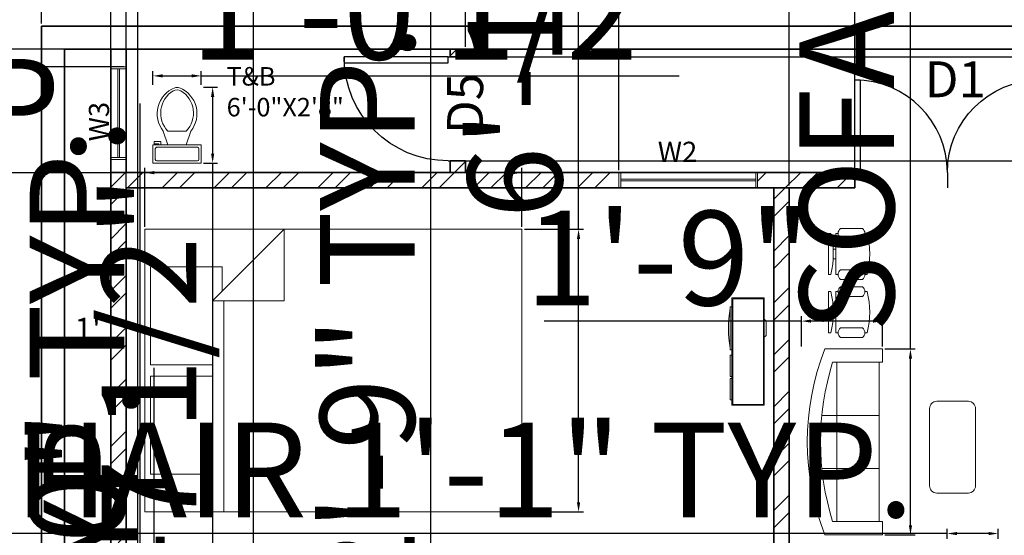
# Model space of a CAD drawing. Units: inches. Extents: x 1542 to 2523, y 1699 to 2449.
# Tile 4 of 7: x 1875 to 2130, y 2158 to 2292. Entities that reach past the tile are written whole.
import ezdxf

# ---------------------------------------------------------------- set-up
doc = ezdxf.new("R2010")
doc.units = ezdxf.units.IN
for name, color, linetype, lineweight in [('A-ANNO-DIMS', 7, 'Continuous', 18), ('A-ANNO-TEXT', 1, 'Continuous', 18), ('A-AREA-IDEN', 1, 'Continuous', 25), ('A-FLOR-FIXT', 9, 'Continuous', 18), ('A-WALL-PATT', 9, 'Continuous', 13), ('doors', 5, 'Continuous', 25), ('furniture', 9, 'Continuous', 18), ('walls', 7, 'Continuous', 35), ('windows', 93, 'Continuous', 18)]:
    doc.layers.add(name, color=color, linetype=linetype, lineweight=lineweight)
doc.styles.get("Standard").update_dxf_attribs({"font": 'arial.ttf'})
doc.dimstyles.new('ISO-25', dxfattribs={"dimtxt": 24.5625, "dimasz": 2.5, "dimexe": 1.25, "dimexo": 0.625, "dimtad": 1, "dimlunit": 4, "dimtxsty": 'Standard', "dimcen": 2.5, "dimadec": 0, "dimazin": 0, "dimtfac": 10, "dimtmove": 0, "dimatfit": 3, "dimfxl": 1, "dimarcsym": 0})

# ---------------------------------------------------------------- blocks, each defined once
blk = doc.blocks.new('*U2')
for p, q in [((0, 0), (0, -5)), ((30, 0), (30, -5))]:
    blk.add_line(p, q)
blk.add_lwpolyline([(0, 0), (0, 30), (1.75, 30), (1.75, 0)], close=True)
blk.add_arc((0, 0), 30, 0, 90)
blk = doc.blocks.new('Sofa - Roundback 7 ft.')
for p, q in [((-12.00002, -32.4421), (-12.00003, -6.5971)), ((11.99997, -32.4421), (11.99998, -6.5971)), ((-36.000027, -34), (-36.000027, -11.4696)), ((35.99998, -34), (35.99998, -11.4696)), ((-35.999844, -13.3819), (35.9998, -13.3819)), ((-36.000027, -32.4421), (35.99998, -32.4421))]:
    blk.add_line(p, q)
for points in [[(-36.000027, -34), (-42.000027, -34), (-42.000027, -8)], [(41.99998, -8), (41.99998, -34), (35.99998, -34)]]:
    blk.add_lwpolyline(points)
for centre, radius, start, end in [((0, -114.25), 114.25, 68.43141, 111.5686), ((-0.00001, -127.1968), 121.1968, 72.72033, 107.2797)]:
    blk.add_arc(centre, radius, start, end)
blk = doc.blocks.new('Bed - Queen')
for p, q in [((0, -80.00003), (0, 0)), ((0, 0), (59.99999, 0)), ((59.99999, 0), (59.99999, -80.00003)), ((7.99999, -1.2), (28.79998, -1.2)), ((7.99999, -14.4), (7.99999, -1.2)), ((28.79998, -1.2), (28.79998, -14.4)), ((31.19999, -1.2), (51.99999, -1.2)), ((31.19999, -14.4), (31.19999, -1.2)), ((51.99999, -1.2), (51.99999, -16.4)), ((0, -14.4), (44.8, -14.4)), ((59.99999, -29.6), (44.8, -14.4)), ((44.8, -14.4), (44.8, -29.6)), ((51.99999, -16.4), (46.79936, -16.4)), ((44.8, -16.8), (0, -16.8)), ((44.8, -29.6), (59.99999, -29.6)), ((59.99999, -80.00003), (0, -80.00003))]:
    blk.add_line(p, q)
blk = doc.blocks.new('Chair - Desk')
for p, q in [((-8.5, 0), (-8.5, -1)), ((-8.5, 0), (8.5, 0)), ((8.5, 0), (8.5, -1)), ((-8.5, -3), (-8.5, -4)), ((-8.5, -3), (8.5, -3)), ((-2, -3), (-2, -1.9355)), ((2, -1.9576), (2, -3)), ((8.5, -3), (8.5, -4)), ((-10.5, -5), (-10.5, -14)), ((-6.5, -14), (-6.5, -5)), ((6.5, -5), (6.5, -14)), ((10.5, -14), (10.5, -5)), ((-8.5, -15), (-8.5, -16)), ((8.5, -15), (8.5, -16))]:
    blk.add_line(p, q)
for centre, radius, start, end in [((-8.5, -6.5), 2.5, 36.8699, 143.1301), ((0, 34.625), 36.625, 256.5803, 283.4197), ((8.5, -6.5), 2.5, 36.8699, 143.1301), ((-8.5, -12.5), 2.5, 216.8699, 323.1301), ((0, 19.625), 36.625, 256.5803, 283.4197), ((8.5, -12.5), 2.5, 216.8699, 323.1301)]:
    blk.add_arc(centre, radius, start, end)
blk = doc.blocks.new('Entertainment Center')
for p, q in [((-4, 0), (-5, -1)), ((4, 0), (-4, 0)), ((5, -1), (4, 0)), ((-17, -19), (-17, -1)), ((-17, -1), (43, -1)), ((-16.5, -18.5), (-16.5, -1.5)), ((-16.5, -1.5), (42.5, -1.5)), ((42.5, -1.5), (42.5, -18.5)), ((43, -1), (43, -19)), ((43, -19), (-17, -19)), ((42.5, -18.5), (-16.5, -18.5)), ((-12, -20), (-12, -19)), ((12, -20), (-12, -20)), ((12, -19), (12, -20)), ((15, -20), (15, -19)), ((27, -20), (15, -20)), ((27, -19), (27, -20)), ((28, -20), (28, -19)), ((40, -20), (28, -20)), ((40, -19), (40, -20))]:
    blk.add_line(p, q)
blk.add_arc((0, 40), 61, 259.6111, 280.3889)
blk = doc.blocks.new('Toilet - top')
for p, q in [((9.5, -6), (9.5, -2)), ((-10, -8.5), (-8, -8.5)), ((-10, -9.5), (-10, -8.5)), ((-8, -8.5), (-8, -8)), ((-7, -8), (-7, -9.5)), ((-4, -8), (-6, -14)), ((4, -8), (6, -14)), ((-7, -9.5), (-10, -9.5)), ((4, -14), (-4, -14))]:
    blk.add_line(p, q)
blk.add_lwpolyline([(10.5, -8), (10.5, 0), (-10.5, 0), (-10.5, -8)], close=True)
for points in [[(-9.5, -2), (-9.5, -6)], [(8.5, -1), (-8.5, -1)], [(-8.5, -7), (8.5, -7)]]:
    blk.add_lwpolyline(points)
for centre, radius, start, end in [((-8.62, -1.88), 0.884, 81.8699, 188.1301), ((8.62, -1.88), 0.884, 351.8699, 98.1301), ((-8.62, -6.12), 0.884, 171.8699, 278.1301), ((8.62, -6.12), 0.884, 261.8699, 8.1301), ((3.52, -21.58), 12.17, 141.4691, 247.9714), ((4.2, -21.82), 11.33, 136.3677, 238.9468), ((-3.52, -21.58), 12.17, 292.0284, 38.5307), ((-4.2, -21.82), 11.33, 301.053, 43.6321), ((0, -27.88), 4, 245.7318, 294.2682), ((0, -29), 4, 254.8605, 285.1395)]:
    blk.add_arc(centre, radius, start, end)
blk = doc.blocks.new('*D9')
at = {"layer": 'A-ANNO-DIMS', "color": 0, "lineweight": -2, "transparency": 16777216}
for p, q in [((1880.38, 2291.06), (1880.38, 2302.87)), ((1882.88, 2301.62), (2237.88, 2301.62)), ((2240.38, 2291.06), (2240.38, 2302.87))]:
    blk.add_line(p, q, dxfattribs=at)
at = {"layer": 'A-ANNO-DIMS', "color": 0, "transparency": 16777216}
for points in [[(1882.88, 2302.04), (1882.88, 2301.2), (1880.38, 2301.62)], [(2237.88, 2302.04), (2237.88, 2301.2), (2240.38, 2301.62)]]:
    blk.add_solid(points, dxfattribs=at)
at = {"layer": 'Defpoints', "color": 0, "transparency": 16777216}
for p in [(2240.38, 2301.62), (1880.38, 2290.44), (2240.38, 2290.44)]:
    blk.add_point(p, dxfattribs=at)
at = {"layer": 'A-ANNO-DIMS', "color": 0, "transparency": 16777216, "insert": (2060.38, 2308.37), "char_height": 12, "attachment_point": 5}
blk.add_mtext("30'", dxfattribs=at)
blk = doc.blocks.new('*D17')
at = {"layer": 'A-ANNO-DIMS', "color": 0, "lineweight": -2, "transparency": 16777216}
for p, q in [((1886.38, 2206.47), (1886.38, 2208.52)), ((1895.88, 2207.27), (1888.88, 2207.27)), ((1898.38, 2206.47), (1898.38, 2208.52))]:
    blk.add_line(p, q, dxfattribs=at)
at = {"layer": 'A-ANNO-DIMS', "color": 0, "transparency": 16777216}
for points in [[(1888.88, 2207.69), (1888.88, 2206.86), (1886.38, 2207.27)], [(1895.88, 2207.69), (1895.88, 2206.86), (1898.38, 2207.27)]]:
    blk.add_solid(points, dxfattribs=at)
at = {"layer": 'Defpoints', "color": 0, "transparency": 16777216}
for p in [(1886.38, 2207.27), (1886.38, 2205.84), (1898.38, 2205.84)]:
    blk.add_point(p, dxfattribs=at)
at = {"layer": 'A-ANNO-DIMS', "color": 0, "transparency": 16777216, "insert": (1892.38, 2210.91), "char_height": 6, "attachment_point": 5}
blk.add_mtext("1'", dxfattribs=at)
blk = doc.blocks.new('WIN-W3-24IN')
for p, q in [((0, 0), (0, 24.03)), ((0, 24.03), (3.94, 24.03)), ((0, 23.53), (3.94, 23.53)), ((1.77, 0.5), (1.77, 23.53)), ((2.17, 0.5), (2.17, 23.53)), ((3.94, 24.03), (3.94, 0)), ((3.94, 0.5), (0, 0.5)), ((3.94, 0), (0, 0))]:
    blk.add_line(p, q)
blk = doc.blocks.new('WIN-W2-36IN')
for p, q in [((0, 3.94), (36.03, 3.94)), ((0, 0), (0, 3.94)), ((0.5, 0), (0.5, 3.94)), ((35.53, 3.94), (35.53, 0)), ((36.03, 3.94), (36.03, 0)), ((36.03, 0), (0, 0)), ((0.5, 2.17), (35.53, 2.17)), ((0.5, 1.77), (35.53, 1.77))]:
    blk.add_line(p, q)
blk = doc.blocks.new('*D26')
at = {"layer": 'A-ANNO-DIMS', "color": 0, "lineweight": -2, "transparency": 16777216}
for p, q in [((2115.34, 2158.69), (1845.86, 2158.69)), ((2115.34, 2157.33), (2115.34, 2159.94)), ((2126.05, 2158.69), (2117.84, 2158.69)), ((2128.55, 2157.33), (2128.55, 2159.94))]:
    blk.add_line(p, q, dxfattribs=at)
at = {"layer": 'A-ANNO-DIMS', "color": 0, "transparency": 16777216}
for points in [[(2117.84, 2159.1), (2117.84, 2158.27), (2115.34, 2158.69)], [(2126.05, 2159.1), (2126.05, 2158.27), (2128.55, 2158.69)]]:
    blk.add_solid(points, dxfattribs=at)
at = {"layer": 'Defpoints', "color": 0, "transparency": 16777216}
for p in [(2115.34, 2158.69), (2115.34, 2156.7), (2128.55, 2156.7)]:
    blk.add_point(p, dxfattribs=at)
at = {"layer": 'A-ANNO-DIMS', "color": 0, "transparency": 16777216, "insert": (1979.35, 2172.01), "char_height": 24.5625, "attachment_point": 5}
blk.add_mtext('CHAIR 1\'-1" TYP.', dxfattribs=at)
blk = doc.blocks.new('*D28')
at = {"layer": 'A-ANNO-DIMS', "color": 0, "lineweight": -2, "transparency": 16777216}
for p, q in [((1905.99, 2054.87), (1905.99, 2270.35)), ((1903.01, 2054.87), (1907.24, 2054.87)), ((1905.99, 2033.33), (1905.99, 2052.37)), ((1903.01, 2030.83), (1907.24, 2030.83))]:
    blk.add_line(p, q, dxfattribs=at)
at = {"layer": 'A-ANNO-DIMS', "color": 0, "transparency": 16777216}
for points in [[(1905.57, 2052.37), (1906.4, 2052.37), (1905.99, 2054.87)], [(1905.57, 2033.33), (1906.4, 2033.33), (1905.99, 2030.83)]]:
    blk.add_solid(points, dxfattribs=at)
at = {"layer": 'Defpoints', "color": 0, "transparency": 16777216}
for p in [(1902.38, 2054.87), (1905.99, 2054.87), (1902.38, 2030.83)]:
    blk.add_point(p, dxfattribs=at)
at = {"layer": 'A-ANNO-DIMS', "color": 0, "transparency": 16777216, "insert": (1892.81, 2163.86), "char_height": 24.5625, "attachment_point": 5, "rotation": 90}
blk.add_mtext('W3 2\'-0" TYP.', dxfattribs=at)
blk = doc.blocks.new('*D30')
at = {"layer": 'A-ANNO-DIMS', "color": 0, "lineweight": -2, "transparency": 16777216}
for p, q in [((2181.19, 2203.89), (2176.38, 2203.89)), ((2177.63, 2201.39), (2177.63, 2178.49)), ((2181.19, 2175.99), (2176.38, 2175.99)), ((2177.63, 2175.99), (2177.63, 1878.93))]:
    blk.add_line(p, q, dxfattribs=at)
at = {"layer": 'A-ANNO-DIMS', "color": 0, "transparency": 16777216}
for points in [[(2177.21, 2201.39), (2178.05, 2201.39), (2177.63, 2203.89)], [(2177.21, 2178.49), (2178.05, 2178.49), (2177.63, 2175.99)]]:
    blk.add_solid(points, dxfattribs=at)
at = {"layer": 'Defpoints', "color": 0, "transparency": 16777216}
for p in [(2181.81, 2203.89), (2177.63, 2175.99), (2181.81, 2175.99)]:
    blk.add_point(p, dxfattribs=at)
at = {"layer": 'A-ANNO-DIMS', "color": 0, "transparency": 16777216, "insert": (2164.46, 2026.21), "char_height": 24.5625, "attachment_point": 5, "rotation": 90}
blk.add_mtext('TV UNIT 2\'-4" TYP.', dxfattribs=at)
blk = doc.blocks.new('*D32')
at = {"layer": 'A-ANNO-DIMS', "color": 0, "lineweight": -2, "transparency": 16777216}
for p, q in [((1922.46, 2274.54), (1926.04, 2274.54)), ((1924.79, 2272.04), (1924.79, 2257.33)), ((1922.46, 2254.83), (1926.04, 2254.83)), ((1924.79, 2254.83), (1924.79, 2060.84))]:
    blk.add_line(p, q, dxfattribs=at)
at = {"layer": 'A-ANNO-DIMS', "color": 0, "transparency": 16777216}
for points in [[(1924.37, 2272.04), (1925.21, 2272.04), (1924.79, 2274.54)], [(1924.37, 2257.33), (1925.21, 2257.33), (1924.79, 2254.83)]]:
    blk.add_solid(points, dxfattribs=at)
at = {"layer": 'Defpoints', "color": 0, "transparency": 16777216}
for p in [(1921.83, 2274.54), (1921.83, 2254.83), (1924.79, 2254.83)]:
    blk.add_point(p, dxfattribs=at)
at = {"layer": 'A-ANNO-DIMS', "color": 0, "transparency": 16777216, "insert": (1911.46, 2156.58), "char_height": 24.5625, "attachment_point": 5, "rotation": 90}
blk.add_mtext('WC 1\'-7 1/2"', dxfattribs=at)
blk = doc.blocks.new('*D33')
at = {"layer": 'A-ANNO-DIMS', "color": 0, "lineweight": -2, "transparency": 16777216}
for p, q in [((1909.3, 2275.17), (1909.3, 2278.75)), ((1921.83, 2275.17), (1921.83, 2278.75)), ((1911.8, 2277.5), (1919.33, 2277.5)), ((1921.83, 2277.5), (2045.8, 2277.5))]:
    blk.add_line(p, q, dxfattribs=at)
at = {"layer": 'A-ANNO-DIMS', "color": 0, "transparency": 16777216}
for points in [[(1911.8, 2277.92), (1911.8, 2277.09), (1909.3, 2277.5)], [(1919.33, 2277.92), (1919.33, 2277.09), (1921.83, 2277.5)]]:
    blk.add_solid(points, dxfattribs=at)
at = {"layer": 'Defpoints', "color": 0, "transparency": 16777216}
for p in [(1921.83, 2277.5), (1909.3, 2274.54), (1921.83, 2274.54)]:
    blk.add_point(p, dxfattribs=at)
at = {"layer": 'A-ANNO-DIMS', "color": 0, "transparency": 16777216, "insert": (1985.06, 2290.83), "char_height": 24.562, "attachment_point": 5}
blk.add_mtext('1\'-0 1/2"', dxfattribs=at)
blk = doc.blocks.new('*D34')
at = {"layer": 'A-ANNO-DIMS', "color": 0, "lineweight": -2, "transparency": 16777216}
for p, q in [((1981.43, 2074.83), (1981.43, 2296.01)), ((1977.09, 2074.83), (1982.68, 2074.83)), ((1981.43, 2044.29), (1981.43, 2072.33)), ((1977.09, 2041.79), (1982.68, 2041.79))]:
    blk.add_line(p, q, dxfattribs=at)
at = {"layer": 'A-ANNO-DIMS', "color": 0, "transparency": 16777216}
for points in [[(1981.01, 2072.33), (1981.84, 2072.33), (1981.43, 2074.83)], [(1981.01, 2044.29), (1981.84, 2044.29), (1981.43, 2041.79)]]:
    blk.add_solid(points, dxfattribs=at)
at = {"layer": 'Defpoints', "color": 0, "transparency": 16777216}
for p in [(1976.47, 2074.83), (1981.43, 2074.83), (1976.47, 2041.79)]:
    blk.add_point(p, dxfattribs=at)
at = {"layer": 'A-ANNO-DIMS', "color": 0, "transparency": 16777216, "insert": (1968.1, 2186.67), "char_height": 24.5625, "attachment_point": 5, "rotation": 90}
blk.add_mtext('WC 2\'-9" TYP.', dxfattribs=at)
blk = doc.blocks.new('*D38')
at = {"layer": 'A-ANNO-DIMS', "color": 0, "lineweight": -2, "transparency": 16777216}
for p, q in [((1907.17, 2238.32), (1907.17, 2253.62)), ((2005.03, 2238.32), (2005.03, 2253.62)), ((1907.17, 2252.37), (1542.11, 2252.37)), ((2002.53, 2252.37), (1909.67, 2252.37))]:
    blk.add_line(p, q, dxfattribs=at)
at = {"layer": 'A-ANNO-DIMS', "color": 0, "transparency": 16777216}
for points in [[(1909.67, 2252.79), (1909.67, 2251.95), (1907.17, 2252.37)], [(2002.53, 2252.79), (2002.53, 2251.95), (2005.03, 2252.37)]]:
    blk.add_solid(points, dxfattribs=at)
at = {"layer": 'Defpoints', "color": 0, "transparency": 16777216}
for p in [(1907.17, 2252.37), (1907.17, 2237.69), (2005.03, 2237.69)]:
    blk.add_point(p, dxfattribs=at)
at = {"layer": 'A-ANNO-DIMS', "color": 0, "transparency": 16777216, "insert": (1723.39, 2266.45), "char_height": 24.5625, "attachment_point": 5}
blk.add_mtext('QUEEN BED 8\'-2" TYP.', dxfattribs=at)
blk = doc.blocks.new('*D39')
at = {"layer": 'A-ANNO-DIMS', "color": 0, "lineweight": -2, "transparency": 16777216}
for p, q in [((2019.71, 2237.69), (2019.71, 2448.53)), ((2005.65, 2237.69), (2020.96, 2237.69)), ((2019.71, 2166.8), (2019.71, 2235.19)), ((2005.65, 2164.3), (2020.96, 2164.3))]:
    blk.add_line(p, q, dxfattribs=at)
at = {"layer": 'A-ANNO-DIMS', "color": 0, "transparency": 16777216}
for points in [[(2019.29, 2235.19), (2020.12, 2235.19), (2019.71, 2237.69)], [(2019.29, 2166.8), (2020.12, 2166.8), (2019.71, 2164.3)]]:
    blk.add_solid(points, dxfattribs=at)
at = {"layer": 'Defpoints', "color": 0, "transparency": 16777216}
for p in [(2005.03, 2237.69), (2019.71, 2237.69), (2005.03, 2164.3)]:
    blk.add_point(p, dxfattribs=at)
at = {"layer": 'A-ANNO-DIMS', "color": 0, "transparency": 16777216, "insert": (2006.38, 2344.36), "char_height": 24.5625, "attachment_point": 5, "rotation": 90}
blk.add_mtext('6\'-1 1/2" TYP.', dxfattribs=at)
blk = doc.blocks.new('*D40')
at = {"layer": 'A-ANNO-DIMS', "color": 0, "lineweight": -2, "transparency": 16777216}
for p, q in [((1909.59, 1986.22), (1909.59, 2201.7)), ((1903.01, 1986.22), (1910.84, 1986.22)), ((1909.59, 1940.69), (1909.59, 1983.72)), ((1903.01, 1938.19), (1910.84, 1938.19))]:
    blk.add_line(p, q, dxfattribs=at)
at = {"layer": 'A-ANNO-DIMS', "color": 0, "transparency": 16777216}
for points in [[(1909.17, 1983.72), (1910, 1983.72), (1909.59, 1986.22)], [(1909.17, 1940.69), (1910, 1940.69), (1909.59, 1938.19)]]:
    blk.add_solid(points, dxfattribs=at)
at = {"layer": 'Defpoints', "color": 0, "transparency": 16777216}
for p in [(1902.38, 1986.22), (1909.59, 1986.22), (1902.38, 1938.19)]:
    blk.add_point(p, dxfattribs=at)
at = {"layer": 'A-ANNO-DIMS', "color": 0, "transparency": 16777216, "insert": (1896.42, 2095.21), "char_height": 24.5625, "attachment_point": 5, "rotation": 90}
blk.add_mtext('W1 4\'-0" TYP.', dxfattribs=at)
blk = doc.blocks.new('*D44')
at = {"layer": 'A-ANNO-DIMS', "color": 0, "lineweight": -2, "transparency": 16777216}
for p, q in [((2105.8, 2206.61), (2105.8, 2435.72)), ((2099.19, 2206.61), (2107.05, 2206.61)), ((2105.8, 2160.85), (2105.8, 2204.11)), ((2099.19, 2158.35), (2107.05, 2158.35))]:
    blk.add_line(p, q, dxfattribs=at)
at = {"layer": 'A-ANNO-DIMS', "color": 0, "transparency": 16777216}
for points in [[(2105.39, 2204.11), (2106.22, 2204.11), (2105.8, 2206.61)], [(2105.39, 2160.85), (2106.22, 2160.85), (2105.8, 2158.35)]]:
    blk.add_solid(points, dxfattribs=at)
at = {"layer": 'Defpoints', "color": 0, "transparency": 16777216}
for p in [(2098.56, 2206.61), (2105.8, 2206.61), (2098.56, 2158.35)]:
    blk.add_point(p, dxfattribs=at)
at = {"layer": 'A-ANNO-DIMS', "color": 0, "transparency": 16777216, "insert": (2092.47, 2322.42), "char_height": 24.5625, "attachment_point": 5, "rotation": 90}
blk.add_mtext('SOFA 4\'-0 1/2"', dxfattribs=at)
blk = doc.blocks.new('*D45')
at = {"layer": 'A-ANNO-DIMS', "color": 0, "lineweight": -2, "transparency": 16777216}
for p, q in [((2077.5, 2207.23), (2077.5, 2215.09)), ((2098.56, 2207.23), (2098.56, 2215.09)), ((2077.5, 2213.84), (2010.77, 2213.84)), ((2096.06, 2213.84), (2080, 2213.84))]:
    blk.add_line(p, q, dxfattribs=at)
at = {"layer": 'A-ANNO-DIMS', "color": 0, "transparency": 16777216}
for points in [[(2080, 2214.26), (2080, 2213.43), (2077.5, 2213.84)], [(2096.06, 2214.26), (2096.06, 2213.43), (2098.56, 2213.84)]]:
    blk.add_solid(points, dxfattribs=at)
at = {"layer": 'Defpoints', "color": 0, "transparency": 16777216}
for p in [(2077.5, 2213.84), (2077.5, 2206.61), (2098.56, 2206.61)]:
    blk.add_point(p, dxfattribs=at)
at = {"layer": 'A-ANNO-DIMS', "color": 0, "transparency": 16777216, "insert": (2042.89, 2227.01), "char_height": 24.562, "attachment_point": 5}
blk.add_mtext('1\'-9"', dxfattribs=at)
blk = doc.blocks.new('*D48')
at = {"layer": 'A-ANNO-DIMS', "color": 0, "lineweight": -2, "transparency": 16777216}
for p, q in [((1905.38, 2077.06), (1905.38, 2320.14)), ((1935.38, 2077.06), (1935.38, 2320.14)), ((1907.88, 2318.89), (1932.88, 2318.89)), ((1935.38, 2318.89), (2004.84, 2318.89))]:
    blk.add_line(p, q, dxfattribs=at)
at = {"layer": 'A-ANNO-DIMS', "color": 0, "transparency": 16777216}
for points in [[(1907.88, 2319.31), (1907.88, 2318.47), (1905.38, 2318.89)], [(1932.88, 2319.31), (1932.88, 2318.47), (1935.38, 2318.89)]]:
    blk.add_solid(points, dxfattribs=at)
at = {"layer": 'Defpoints', "color": 0, "transparency": 16777216}
for p in [(1935.38, 2318.89), (1905.38, 2076.44), (1935.38, 2076.44)]:
    blk.add_point(p, dxfattribs=at)
at = {"layer": 'A-ANNO-DIMS', "color": 0, "transparency": 16777216, "insert": (1971.36, 2332.05), "char_height": 24.562, "attachment_point": 5}
blk.add_mtext('2\'-6"', dxfattribs=at)
blk = doc.blocks.new('*D50')
at = {"layer": 'A-ANNO-DIMS', "color": 0, "lineweight": -2, "transparency": 16777216}
for p, q in [((2268.83, 2282.44), (2268.83, 2351.9)), ((1987.01, 2282.44), (2270.08, 2282.44)), ((2268.83, 2257.94), (2268.83, 2279.94)), ((1987.01, 2255.44), (2270.08, 2255.44))]:
    blk.add_line(p, q, dxfattribs=at)
at = {"layer": 'A-ANNO-DIMS', "color": 0, "transparency": 16777216}
for points in [[(2268.42, 2279.94), (2269.25, 2279.94), (2268.83, 2282.44)], [(2268.42, 2257.94), (2269.25, 2257.94), (2268.83, 2255.44)]]:
    blk.add_solid(points, dxfattribs=at)
at = {"layer": 'Defpoints', "color": 0, "transparency": 16777216}
for p in [(1986.38, 2282.44), (2268.83, 2282.44), (1986.38, 2255.44)]:
    blk.add_point(p, dxfattribs=at)
at = {"layer": 'A-ANNO-DIMS', "color": 0, "transparency": 16777216, "insert": (2255.66, 2318.42), "char_height": 24.562, "attachment_point": 5, "rotation": 90}
blk.add_mtext('2\'-3"', dxfattribs=at)
blk = doc.blocks.new('*D57')
at = {"layer": 'A-ANNO-DIMS', "color": 0, "lineweight": -2, "transparency": 16777216}
for p, q in [((1851.93, 2089.65), (1851.93, 2178.19)), ((1897.82, 2089.65), (1850.68, 2089.65)), ((1851.93, 2057.37), (1851.93, 2087.15)), ((1897.82, 2054.87), (1850.68, 2054.87))]:
    blk.add_line(p, q, dxfattribs=at)
at = {"layer": 'A-ANNO-DIMS', "color": 0, "transparency": 16777216}
for points in [[(1851.52, 2087.15), (1852.35, 2087.15), (1851.93, 2089.65)], [(1851.52, 2057.37), (1852.35, 2057.37), (1851.93, 2054.87)]]:
    blk.add_solid(points, dxfattribs=at)
at = {"layer": 'Defpoints', "color": 0, "transparency": 16777216}
for p in [(1851.93, 2089.65), (1898.45, 2089.65), (1898.45, 2054.87)]:
    blk.add_point(p, dxfattribs=at)
at = {"layer": 'A-ANNO-DIMS', "color": 0, "transparency": 16777216, "insert": (1838.98, 2135.17), "char_height": 24.562, "attachment_point": 5, "rotation": 90}
blk.add_mtext('2\'-11"', dxfattribs=at)
blk = doc.blocks.new('*D61')
at = {"layer": 'A-ANNO-DIMS', "color": 0, "lineweight": -2, "transparency": 16777216}
for p, q in [((1898.38, 2253.06), (1898.38, 2320.14)), ((2030.14, 2253.06), (2030.14, 2320.14)), ((1900.88, 2318.89), (2027.64, 2318.89))]:
    blk.add_line(p, q, dxfattribs=at)
at = {"layer": 'A-ANNO-DIMS', "color": 0, "transparency": 16777216}
for points in [[(1900.88, 2319.31), (1900.88, 2318.47), (1898.38, 2318.89)], [(2027.64, 2319.31), (2027.64, 2318.47), (2030.14, 2318.89)]]:
    blk.add_solid(points, dxfattribs=at)
at = {"layer": 'Defpoints', "color": 0, "transparency": 16777216}
for p in [(2030.14, 2318.89), (1898.38, 2252.44), (2030.14, 2252.44)]:
    blk.add_point(p, dxfattribs=at)
at = {"layer": 'A-ANNO-DIMS', "color": 0, "transparency": 16777216, "insert": (1964.26, 2332.05), "char_height": 24.562, "attachment_point": 5}
blk.add_mtext('11\'-0"', dxfattribs=at)
blk = doc.blocks.new('*D62')
at = {"layer": 'A-ANNO-DIMS', "color": 0, "lineweight": -2, "transparency": 16777216}
for p, q in [((2074.38, 2249.06), (2074.38, 2320.14)), ((2091.38, 2249.06), (2091.38, 2320.14)), ((2076.88, 2318.89), (2088.88, 2318.89)), ((2091.38, 2318.89), (2158.11, 2318.89))]:
    blk.add_line(p, q, dxfattribs=at)
at = {"layer": 'A-ANNO-DIMS', "color": 0, "transparency": 16777216}
for points in [[(2076.88, 2319.31), (2076.88, 2318.47), (2074.38, 2318.89)], [(2088.88, 2319.31), (2088.88, 2318.47), (2091.38, 2318.89)]]:
    blk.add_solid(points, dxfattribs=at)
at = {"layer": 'Defpoints', "color": 0, "transparency": 16777216}
for p in [(2091.38, 2318.89), (2074.38, 2248.44), (2091.38, 2248.44)]:
    blk.add_point(p, dxfattribs=at)
at = {"layer": 'A-ANNO-DIMS', "color": 0, "transparency": 16777216, "insert": (2126, 2332.05), "char_height": 24.562, "attachment_point": 5}
blk.add_mtext('1\'-5"', dxfattribs=at)
blk = doc.blocks.new('*D65')
at = {"layer": 'A-ANNO-DIMS', "color": 0, "lineweight": -2, "transparency": 16777216}
for p, q in [((1898.38, 2285.06), (1898.38, 2320.14)), ((1990.38, 2285.06), (1990.38, 2320.14)), ((1900.88, 2318.89), (1987.88, 2318.89))]:
    blk.add_line(p, q, dxfattribs=at)
at = {"layer": 'A-ANNO-DIMS', "color": 0, "transparency": 16777216}
for points in [[(1900.88, 2319.31), (1900.88, 2318.47), (1898.38, 2318.89)], [(1987.88, 2319.31), (1987.88, 2318.47), (1990.38, 2318.89)]]:
    blk.add_solid(points, dxfattribs=at)
at = {"layer": 'Defpoints', "color": 0, "transparency": 16777216}
for p in [(1990.38, 2318.89), (1898.38, 2284.44), (1990.38, 2284.44)]:
    blk.add_point(p, dxfattribs=at)
at = {"layer": 'A-ANNO-DIMS', "color": 0, "transparency": 16777216, "insert": (1944.38, 2332.05), "char_height": 24.562, "attachment_point": 5}
blk.add_mtext('7\'-8"', dxfattribs=at)
blk = doc.blocks.new('*D66')
at = {"layer": 'A-ANNO-DIMS', "color": 0, "lineweight": -2, "transparency": 16777216}
for p, q in [((1851.93, 2286.94), (1851.93, 2413.22)), ((1901.76, 2284.44), (1850.68, 2284.44)), ((1851.93, 2279.86), (1851.93, 2284.44)), ((1901.76, 2279.86), (1850.68, 2279.86)), ((1851.93, 2277.36), (1851.93, 2274.86))]:
    blk.add_line(p, q, dxfattribs=at)
at = {"layer": 'A-ANNO-DIMS', "color": 0, "transparency": 16777216}
for points in [[(1851.52, 2286.94), (1852.35, 2286.94), (1851.93, 2284.44)], [(1851.52, 2277.36), (1852.35, 2277.36), (1851.93, 2279.86)]]:
    blk.add_solid(points, dxfattribs=at)
at = {"layer": 'Defpoints', "color": 0, "transparency": 16777216}
for p in [(1851.93, 2284.44), (1902.38, 2284.44), (1902.38, 2279.86)]:
    blk.add_point(p, dxfattribs=at)
at = {"layer": 'A-ANNO-DIMS', "color": 0, "transparency": 16777216, "insert": (1838.61, 2351.33), "char_height": 24.562, "attachment_point": 5, "rotation": 90}
blk.add_mtext('0\'-4 1/2"', dxfattribs=at)
blk = doc.blocks.new('*D69')
at = {"layer": 'A-ANNO-DIMS', "color": 0, "lineweight": -2, "transparency": 16777216}
for p, q in [((1902.38, 2077.06), (1902.38, 2320.14)), ((1905.38, 2077.06), (1905.38, 2320.14)), ((1899.88, 2318.89), (1897.38, 2318.89)), ((1902.38, 2318.89), (1905.38, 2318.89)), ((1907.88, 2318.89), (1976.93, 2318.89))]:
    blk.add_line(p, q, dxfattribs=at)
at = {"layer": 'A-ANNO-DIMS', "color": 0, "transparency": 16777216}
for points in [[(1899.88, 2319.31), (1899.88, 2318.47), (1902.38, 2318.89)], [(1907.88, 2319.31), (1907.88, 2318.47), (1905.38, 2318.89)]]:
    blk.add_solid(points, dxfattribs=at)
at = {"layer": 'Defpoints', "color": 0, "transparency": 16777216}
for p in [(1905.38, 2318.89), (1902.38, 2076.44), (1905.38, 2076.44)]:
    blk.add_point(p, dxfattribs=at)
at = {"layer": 'A-ANNO-DIMS', "color": 0, "transparency": 16777216, "insert": (1943.65, 2332.06), "char_height": 24.562, "attachment_point": 5}
blk.add_mtext('0\'-3"', dxfattribs=at)

msp = doc.modelspace()

# ---------------------------------------------------------------- hatches: boundary and pattern name
at = {"layer": 'A-WALL-PATT'}
h = msp.add_hatch(dxfattribs=at)
h.set_pattern_fill('ANSI32', color=256)
h.paths.add_polyline_path([(1902.383, 2284.439), (1898.383, 2284.439), (1898.383, 2252.439), (1902.383, 2252.439), (1902.383, 2255.826), (1898.446, 2255.826), (1898.446, 2279.859), (1902.383, 2279.859)])
h = msp.add_hatch(dxfattribs=at)
h.set_pattern_fill('ANSI32', color=256)
h.paths.add_polyline_path([(1990.383, 2282.439), (1990.383, 2284.439), (1986.383, 2284.439), (1986.383, 2282.439)])
h = msp.add_hatch(dxfattribs=at)
h.set_pattern_fill('ANSI32', color=256)
h.paths.add_polyline_path([(1902.383, 2255.826), (1898.383, 2255.826), (1898.383, 2252.439), (1902.383, 2252.439)], flags=17)
h = msp.add_hatch(dxfattribs=at)
h.set_pattern_fill('ANSI32', color=256)
h.paths.add_polyline_path([(1990.383, 2255.439), (1986.383, 2255.439), (1986.383, 2252.439), (1990.383, 2252.439)])
h = msp.add_hatch(dxfattribs=at)
h.set_pattern_fill('ANSI32', color=256)
h.paths.add_polyline_path([(1902.383, 2125.681), (1898.383, 2125.681), (1898.383, 2252.439), (2030.138, 2252.439), (2030.138, 2248.439), (1902.383, 2248.439)])
h = msp.add_hatch(dxfattribs=at)
h.set_pattern_fill('ANSI32', color=256)
h.paths.add_polyline_path([(2091.383, 2252.439), (2066.17, 2252.439), (2066.17, 2248.439), (2091.383, 2248.439)])
h = msp.add_hatch(dxfattribs=at)
h.set_pattern_fill('ANSI32', color=256)
h.paths.add_polyline_path([(2074.383, 2248.439), (2070.383, 2248.439), (2070.383, 2119.439), (2074.383, 2119.439)])

# ---------------------------------------------------------------- linework, layer by layer
at = {"layer": 'furniture'}
msp.add_lwpolyline([(2110.762, 2191.173, -0.4142136), (2112.613, 2193.025), (2120.82, 2193.025, -0.4142136), (2122.671, 2191.173), (2122.671, 2171.058, -0.4142136), (2120.82, 2169.206), (2112.613, 2169.206, -0.4142136), (2110.762, 2171.058)], format="xyb", close=True, dxfattribs=at)
at = {"layer": 'walls'}
for p, q in [((1880.383, 2290.439), (2240.383, 2290.439)), ((1880.383, 1750.439), (1880.383, 2290.439)), ((1886.383, 2284.439), (2234.383, 2284.439)), ((1886.383, 1756.439), (1886.383, 2284.439)), ((1898.383, 2252.439), (1898.383, 2284.439)), ((1902.383, 2252.439), (1902.383, 2284.439)), ((1986.383, 2282.439), (1986.383, 2284.439)), ((1990.383, 2284.439), (1990.383, 2282.439)), ((1990.383, 2282.439), (1990.383, 2284.439)), ((1990.383, 2282.439), (1986.383, 2282.439)), ((1986.383, 2252.439), (1986.383, 2255.439)), ((1986.383, 2255.439), (1990.383, 2255.439)), ((1990.383, 2252.439), (1990.383, 2255.439)), ((1898.383, 1840.439), (1898.383, 2252.439)), ((2091.383, 2252.439), (1898.383, 2252.439)), ((2091.383, 2248.439), (2091.383, 2252.439)), ((1902.383, 1844.439), (1902.383, 2248.439)), ((2091.383, 2248.439), (1902.383, 2248.439)), ((2070.383, 2119.439), (2070.383, 2248.439)), ((2074.383, 2119.439), (2074.383, 2248.439))]:
    msp.add_line(p, q, dxfattribs=at)

# ---------------------------------------------------------------- block references
at = {"layer": 'A-FLOR-FIXT', "xscale": -0.596708182801364, "yscale": 0.596708182801364, "zscale": 0.596708182801364, "rotation": 180}
msp.add_blockref('Toilet - top', (1915.565, 2254.826), dxfattribs=at)
at = {"layer": 'doors', "xscale": -0.9000000000000001, "yscale": 0.9000000000000001, "zscale": 0.9000000000000001, "rotation": 90}
msp.add_blockref('*U2', (1985.883, 2282.439), dxfattribs=at)
at = {"layer": 'doors', "yscale": 0.8, "zscale": 0.8}
for p, xscale in [((2091.383, 2252.439), 0.8), ((2139.383, 2252.439), -0.8)]:
    msp.add_blockref('*U2', p, dxfattribs=dict(at, xscale=xscale))
at = {"layer": 'furniture'}
for name, p, xscale, yscale, zscale, rotation in [('Bed - Queen', (1907.173, 2164.301), 1.223193858347369, 1.223193858347369, 1.223193858347369, 90), ('Chair - Desk', (2084.536, 2231.268), 0.6288640780466365, 0.6288640780466365, 0.6288640780466365, 89.99999999999999), ('Chair - Desk', (2084.536, 2216.154), 0.6288640780466365, 0.6288640780466365, 0.6288640780466365, 89.99999999999999), ('Entertainment Center', (2068.339, 2211.979), 0.4648726153281338, 0.4648726153281338, 0.4648726153281338, 270), ('Sofa - Roundback 7 ft.', (2079.034, 2182.48), 0.5744311325725425, 0.5744311325725425, 0.5744311325725425, 89.99999999999999)]:
    msp.add_blockref(name, p, dxfattribs=dict(at, xscale=xscale, yscale=yscale, zscale=zscale, rotation=rotation))
at = {"layer": 'windows', "rotation": 180}
msp.add_blockref('WIN-W3-24IN', (1902.383, 2279.859), dxfattribs=at)
at = {"layer": 'windows'}
msp.add_blockref('WIN-W2-36IN', (2030.138, 2248.502), dxfattribs=at)

# ---------------------------------------------------------------- texts
at = {"layer": 'A-ANNO-TEXT', "attachment_point": 1}
for s, width, gutter_width, insert, char_height in [('D1', 3.38383, 46.636, (2109.517, 2281.279), 9.3273), ('W2', 1.62225, 26.164, (2040.269, 2260.399), 5.2329)]:
    msp.add_mtext_dynamic_manual_height_columns(s, width=width, gutter_width=gutter_width, heights=[0], dxfattribs=dict(at, insert=insert, char_height=char_height))
at = {"layer": 'A-ANNO-TEXT', "attachment_point": 1, "rotation": 90}
for s, width, gutter_width, insert, char_height in [('D5', 3.38383, 46.636, (1985.614, 2262.416), 9.3273), ('W3', 1.62225, 26.164, (1892.694, 2260.518), 5.2329)]:
    msp.add_mtext_dynamic_manual_height_columns(s, width=width, gutter_width=gutter_width, heights=[0], dxfattribs=dict(at, insert=insert, char_height=char_height))
at = {"layer": 'A-AREA-IDEN', "insert": (1928.428, 2279.781), "char_height": 4.7977, "attachment_point": 1}
msp.add_mtext_dynamic_manual_height_columns('T&B\\P6\'-0"X2\'8"', width=3.29417, gutter_width=23.989, heights=[0], dxfattribs=at)

# ---------------------------------------------------------------- dimensions: what is measured, and where the dimension line sits
at = {"layer": 'A-ANNO-DIMS'}
for base, p1, p2, angle, text, picture, middle in [((2019.707, 2237.692), (2005.029, 2164.301), (2005.029, 2237.692), 90, '<> TYP.', '*D39', (2006.382, 2344.362)), ((2105.802, 2206.606), (2098.565, 2158.354), (2098.565, 2206.606), 90, 'SOFA <>', '*D44', (2092.469, 2322.416)), ((1907.173, 2252.371), (2005.029, 2237.692), (1907.173, 2237.692), 180, 'QUEEN BED <> TYP.', '*D38', (1723.39, 2266.45)), ((1981.426, 2074.834), (1976.469, 2041.788), (1976.469, 2074.834), 90, 'WC <> TYP.', '*D34', (1968.101, 2186.673)), ((1924.788, 2254.826), (1921.831, 2274.545), (1921.831, 2254.826), 270, 'WC <>', '*D32', (1911.463, 2156.584)), ((1905.987, 2054.866), (1902.383, 2030.833), (1902.383, 2054.866), 90, 'W3 <> TYP.', '*D28', (1892.813, 2163.856)), ((2115.34, 2158.686), (2128.547, 2156.705), (2115.34, 2156.705), 180, 'CHAIR <> TYP.', '*D26', (1979.35, 2172.011)), ((1909.587, 1986.223), (1902.383, 1938.191), (1902.383, 1986.223), 90, 'W1 <> TYP.', '*D40', (1896.422, 2095.213)), ((2177.629, 2175.993), (2181.813, 2203.885), (2181.813, 2175.993), 270, 'TV UNIT <> TYP.', '*D30', (2164.463, 2026.213))]:
    dim = msp.add_linear_dim(base=base, p1=p1, p2=p2, angle=angle, text=text, dimstyle='ISO-25', override={"dimdec": 1, "dimlfac": 1, "dimrnd": 0, "dimzin": 1, "dimdsep": 46, "dimlunit": 4, "dimfrac": 2}, dxfattribs=at)
    dim.commit()
    dim.dimension.update_dxf_attribs({"geometry": picture, "text_midpoint": middle})
for base, p1, p2, angle, picture, middle in [((1851.933, 2284.439), (1902.383, 2279.859), (1902.383, 2284.439), 90, '*D66', (1838.607, 2351.328)), ((2268.833, 2282.439), (1986.383, 2255.439), (1986.383, 2282.439), 90, '*D50', (2255.658, 2318.42)), ((2077.502, 2213.844), (2098.565, 2206.606), (2077.502, 2206.606), 180, '*D45', (2042.887, 2227.01)), ((1851.933, 2089.649), (1898.446, 2054.866), (1898.446, 2089.649), 90, '*D57', (1838.976, 2135.172))]:
    dim = msp.add_linear_dim(base=base, p1=p1, p2=p2, angle=angle, dimstyle='ISO-25', override={"dimdec": 1, "dimlfac": 1, "dimrnd": 0, "dimzin": 1, "dimdsep": 46, "dimlunit": 4, "dimfrac": 2}, dxfattribs=at)
    dim.commit()
    dim.dimension.update_dxf_attribs({"geometry": picture, "text_midpoint": middle})
for base, p1, p2, override, picture, middle in [((1905.383, 2318.889), (1902.383, 2076.439), (1905.383, 2076.439), {"dimdec": 1, "dimlfac": 1, "dimrnd": 0, "dimzin": 1, "dimdsep": 46, "dimlunit": 4, "dimfrac": 2}, '*D69', (1943.654, 2332.063)), ((2030.138, 2318.889), (1898.383, 2252.439), (2030.138, 2252.439), {"dimdec": 1, "dimlfac": 1, "dimrnd": 0, "dimzin": 1, "dimdsep": 46, "dimlunit": 4, "dimfrac": 2}, '*D61', (1964.26, 2332.055)), ((1990.383, 2318.889), (1898.383, 2284.439), (1990.383, 2284.439), {"dimdec": 1, "dimlfac": 1, "dimrnd": 0, "dimzin": 1, "dimdsep": 46, "dimlunit": 4, "dimfrac": 2}, '*D65', (1944.383, 2332.055)), ((1935.383, 2318.889), (1905.383, 2076.439), (1935.383, 2076.439), {"dimdec": 1, "dimlfac": 1, "dimrnd": 0, "dimzin": 1, "dimdsep": 46, "dimlunit": 4, "dimfrac": 2}, '*D48', (1971.364, 2332.055)), ((2091.383, 2318.889), (2074.383, 2248.439), (2091.383, 2248.439), {"dimdec": 1, "dimlfac": 1, "dimrnd": 0, "dimzin": 1, "dimdsep": 46, "dimlunit": 4, "dimfrac": 2}, '*D62', (2125.998, 2332.055)), ((1921.831, 2277.503), (1909.3, 2274.545), (1921.831, 2274.545), {"dimdec": 1, "dimlfac": 1, "dimrnd": 0, "dimzin": 1, "dimdsep": 46, "dimlunit": 4, "dimfrac": 2}, '*D33', (1985.063, 2290.828)), ((2240.383, 2301.619), (1880.383, 2290.439), (2240.383, 2290.439), {"dimtxt": 12, "dimclrd": 0, "dimclre": 0, "dimclrt": 0}, '*D9', (2060.383, 2308.375)), ((1886.383, 2207.273), (1898.383, 2205.844), (1886.383, 2205.844), {"dimtxt": 6, "dimclrd": 0, "dimclre": 0, "dimclrt": 0}, '*D17', (1892.383, 2210.91))]:
    dim = msp.add_linear_dim(base=base, p1=p1, p2=p2, dimstyle='ISO-25', override=override, dxfattribs=at)
    dim.commit()
    dim.dimension.update_dxf_attribs({"geometry": picture, "text_midpoint": middle})

doc.saveas('drawing.dxf')
